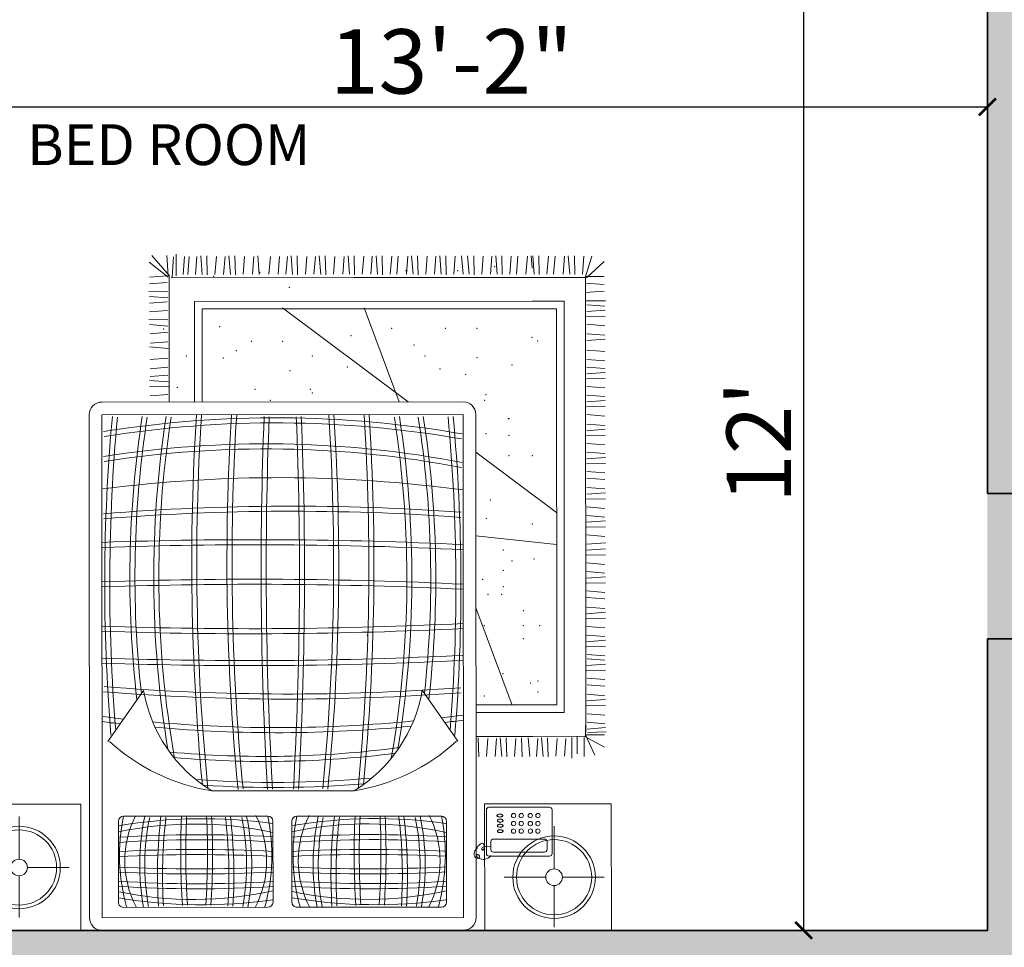
# Model space of a CAD drawing. Units: inches. Extents: x 1704 to 2334, y 1856 to 2559.
# Tile 5 of 10: x 1779 to 1925, y 2353 to 2489. Entities that reach past the tile are written whole.
import ezdxf

# ---------------------------------------------------------------- set-up
doc = ezdxf.new("R2010")
doc.units = ezdxf.units.IN
for name, color, linetype, lineweight in [('A-ANNO-DIMS', 2, 'Continuous', 18), ('A-AREA-IDEN', 7, 'Continuous', 18), ('A-WALL', 7, 'Continuous', 35), ('BEDS', 17, 'Continuous', 18)]:
    doc.layers.add(name, color=color, linetype=linetype, lineweight=lineweight)
doc.layers.add('A-WALL-PATT', color=18, linetype='Continuous', lineweight=13, true_color=0x000000)
doc.styles.get("Standard").update_dxf_attribs({"font": 'arial.ttf'})
doc.dimstyles.new('ISO-25', dxfattribs={"dimtxt": 9.5, "dimasz": 2.5, "dimexe": 1.25, "dimexo": 0.625, "dimtad": 1, "dimdec": 0, "dimlunit": 4, "dimtxsty": 'Standard', "dimblk": 'ARCHTICK', "dimcen": 2.5, "dimse1": 1, "dimse2": 1, "dimclrd": 3, "dimadec": 0, "dimazin": 0, "dimtfac": 1, "dimtdec": 0, "dimtmove": 0, "dimatfit": 3, "dimfxl": 1, "dimarcsym": 0})

# ---------------------------------------------------------------- blocks, each defined once
blk = doc.blocks.new('A$C77DF40FE')
for p, q in [((0.5, 2.6723), (0, 2.6723)), ((0, 2.6723), (0, 2.1723)), ((0.226, 2.4949), (0.226, 2.6594)), ((0.5, 2.1723), (0.5, 2.6723)), ((0.5839, 2.6714), (2.0097, 2.6714)), ((2.0936, 2.1723), (2.0936, 2.6723)), ((2.0936, 2.6723), (2.5936, 2.6723)), ((2.5936, 2.6723), (2.5936, 2.1723)), ((0.5339, 0.6344), (0.5339, 2.6214)), ((0.5839, 2.6214), (2.0097, 2.6214)), ((0.5839, 0.6344), (0.5839, 2.6214)), ((2.0097, 2.6214), (2.0097, 0.6344)), ((2.0597, 2.6214), (2.0597, 0.6344)), ((2.3379, 2.4554), (2.3379, 2.6199)), ((1.2408, 2.5803), (0.6708, 2.5803)), ((1.9255, 2.5803), (1.3555, 2.5803)), ((0.6508, 2.5603), (0.6508, 2.2403)), ((1.2608, 2.2403), (1.2608, 2.5603)), ((1.3355, 2.5603), (1.3355, 2.2403)), ((1.9455, 2.2403), (1.9455, 2.5603)), ((0.0287, 2.4621), (0.1932, 2.4621)), ((0.2588, 2.4621), (0.4233, 2.4621)), ((0.226, 2.261), (0.226, 2.4293)), ((2.3051, 2.4226), (2.1406, 2.4226)), ((2.5352, 2.4226), (2.3707, 2.4226)), ((0.4828, 2.3788, 10.4), (0.2438, 2.3788, 10.4)), ((0.4809, 2.3823), (0.4746, 2.3757)), ((0.4873, 2.387), (0.4809, 2.3823)), ((0.4937, 2.3899), (0.4873, 2.387)), ((0.5, 2.3914), (0.4937, 2.3899)), ((0.506, 2.3917), (0.5, 2.3914)), ((0.5117, 2.391), (0.506, 2.3917)), ((0.5168, 2.3897), (0.5117, 2.391)), ((0.5212, 2.3878), (0.5168, 2.3897)), ((0.5205, 2.3816), (0.5202, 2.3804)), ((0.5202, 2.3804), (0.5202, 2.379)), ((0.5202, 2.379), (0.5206, 2.3777)), ((0.521, 2.3828), (0.5205, 2.3816)), ((0.5206, 2.3777), (0.5213, 2.3764)), ((0.5219, 2.3839), (0.521, 2.3828)), ((0.5248, 2.3858), (0.5212, 2.3878)), ((0.5213, 2.3764), (0.5224, 2.3752)), ((0.523, 2.3849), (0.5219, 2.3839)), ((0.5224, 2.3752), (0.5237, 2.374)), ((0.5244, 2.3856), (0.523, 2.3849)), ((0.5237, 2.374), (0.5252, 2.3731)), ((0.5261, 2.3861), (0.5244, 2.3856)), ((0.5277, 2.3836), (0.5248, 2.3858)), ((0.5252, 2.3731), (0.5268, 2.3723)), ((0.5279, 2.3864), (0.5261, 2.3861)), ((0.5268, 2.3723), (0.5283, 2.3719)), ((0.5298, 2.3813), (0.5277, 2.3836)), ((0.5298, 2.3864), (0.5279, 2.3864)), ((0.5283, 2.3719), (0.5297, 2.3717)), ((0.5297, 2.3717), (0.531, 2.372)), ((0.5318, 2.3861), (0.5298, 2.3864)), ((0.5313, 2.3792), (0.5298, 2.3813)), ((0.531, 2.372), (0.5319, 2.3726)), ((0.5322, 2.3771), (0.5313, 2.3792)), ((0.5338, 2.3855), (0.5318, 2.3861)), ((0.5319, 2.3726), (0.5325, 2.3738)), ((0.5326, 2.3753), (0.5322, 2.3771)), ((0.5325, 2.3738), (0.5326, 2.3753)), ((0.5356, 2.3846), (0.5338, 2.3855)), ((0.5373, 2.3832), (0.5356, 2.3846)), ((0.5387, 2.3815), (0.5373, 2.3832)), ((0.5399, 2.3794), (0.5387, 2.3815)), ((0.5407, 2.377), (0.5399, 2.3794)), ((0.5412, 2.3743), (0.5407, 2.377)), ((0.5414, 2.3715), (0.5412, 2.3743)), ((0.5413, 2.3686), (0.5414, 2.3715)), ((2.3379, 2.2215), (2.3379, 2.3898)), ((0.2338, 2.3688, 10.4), (0.2338, 2.1957, 10.4)), ((0.2538, 2.353, 10.4), (0.2538, 2.3215, 10.4)), ((0.4656, 2.363, 10.4), (0.2638, 2.363, 10.4)), ((0.4756, 2.3215, 10.4), (0.4756, 2.353, 10.4)), ((0.4767, 2.3409), (0.4876, 2.34)), ((0.4876, 2.34), (0.4961, 2.3402)), ((0.4928, 2.1957, 10.4), (0.4928, 2.3688, 10.4)), ((0.4961, 2.3402), (0.5023, 2.3413)), ((0.502, 2.3463), (0.5017, 2.3431)), ((0.5017, 2.3431), (0.5018, 2.3398)), ((0.5018, 2.3398), (0.5023, 2.3365)), ((0.5026, 2.3491), (0.502, 2.3463)), ((0.5023, 2.3413), (0.5067, 2.3431)), ((0.5023, 2.3365), (0.5031, 2.3334)), ((0.5035, 2.3514), (0.5026, 2.3491)), ((0.5031, 2.3334), (0.5043, 2.3309)), ((0.5047, 2.3531), (0.5035, 2.3514)), ((0.5059, 2.3542), (0.5047, 2.3531)), ((0.5073, 2.3548), (0.5059, 2.3542)), ((0.5067, 2.3431), (0.5095, 2.3452)), ((0.5086, 2.3549), (0.5073, 2.3548)), ((0.5097, 2.3544), (0.5086, 2.3549)), ((0.5095, 2.3452), (0.511, 2.3475)), ((0.5107, 2.3534), (0.5097, 2.3544)), ((0.5113, 2.3518), (0.5107, 2.3534)), ((0.511, 2.3475), (0.5115, 2.3498)), ((0.5115, 2.3498), (0.5113, 2.3518)), ((0.5163, 2.3304), (0.5193, 2.3325)), ((0.5193, 2.3325), (0.5222, 2.3349)), ((0.5222, 2.3349), (0.5249, 2.3374)), ((0.5249, 2.3374), (0.5271, 2.3398)), ((0.5271, 2.3398), (0.5288, 2.3419)), ((0.5288, 2.3419), (0.5299, 2.3436)), ((0.5299, 2.3436), (0.5305, 2.3449)), ((0.53, 2.3482), (0.5302, 2.3488)), ((0.5301, 2.3477), (0.53, 2.3482)), ((0.5303, 2.3472), (0.5301, 2.3477)), ((0.5302, 2.3488), (0.5308, 2.3495)), ((0.5306, 2.3466), (0.5303, 2.3472)), ((0.5305, 2.3449), (0.5307, 2.3459)), ((0.5307, 2.3459), (0.5306, 2.3466)), ((0.5308, 2.3495), (0.5317, 2.3504)), ((0.5317, 2.3504), (0.5329, 2.3515)), ((0.5329, 2.3515), (0.5342, 2.3528)), ((0.5342, 2.3528), (0.5356, 2.3543)), ((0.5356, 2.3543), (0.537, 2.3561)), ((0.537, 2.3561), (0.5383, 2.3581)), ((0.5383, 2.3581), (0.5394, 2.3604)), ((0.5394, 2.3604), (0.5403, 2.3629)), ((0.5403, 2.3629), (0.5409, 2.3657)), ((0.5409, 2.3657), (0.5413, 2.3686)), ((0.2638, 2.3115, 10.4), (0.4656, 2.3115, 10.4)), ((0.5043, 2.3309), (0.506, 2.329)), ((0.506, 2.329), (0.5081, 2.328)), ((0.5081, 2.328), (0.5106, 2.328)), ((0.5106, 2.328), (0.5134, 2.3288)), ((0.5134, 2.3288), (0.5163, 2.3304)), ((0.6708, 2.2203), (1.2408, 2.2203)), ((1.3555, 2.2203), (1.9255, 2.2203)), ((0.2438, 2.1857, 10.4), (0.4828, 2.1857, 10.4)), ((0, 2.1723), (0.5, 2.1723)), ((2.5936, 2.1723), (2.0936, 2.1723)), ((1.5773, 2.1205), (1.0147, 2.1205)), ((0.1072, 1.986), (0.1072, 1.911)), ((0.1554, 1.9914), (0.1554, 1.911)), ((0.1792, 1.9138), (0.1849, 1.9847)), ((0.2134, 1.9138), (0.219, 1.9847)), ((0.251, 1.9118), (0.2494, 1.9865)), ((0.2748, 1.9118), (0.2691, 1.9849)), ((0.2899, 1.9138), (0.2956, 1.9847)), ((0.3277, 1.9118), (0.3219, 1.9849)), ((0.3539, 1.9118), (0.3522, 1.9865)), ((0.3766, 1.9138), (0.3822, 1.9847)), ((0.4142, 1.9118), (0.4126, 1.9865)), ((0.438, 1.9118), (0.4323, 1.9849)), ((0.4531, 1.9138), (0.4588, 1.9847)), ((0.4873, 1.9138), (0.493, 1.9847)), ((0.5249, 1.9118), (0.5233, 1.9865)), ((0.1072, 1.9057), (0.0269, 1.9485)), ((0.0644, 1.9807), (0.1019, 1.9003)), ((0.134, 1.9753), (0.134, 1.9057)), ((0.3112, 1.9057), (0.1019, 1.9057)), ((0.1019, 1.9057), (0.1019, 1.8628)), ((0.5301, 1.9057), (0.3112, 1.9057)), ((0.6051, 1.925), (0.7457, 1.7234)), ((1.9869, 1.925), (1.8463, 1.7234)), ((0.0195, 1.8887), (0.0942, 1.8903)), ((0.0227, 1.8712), (0.0957, 1.8769)), ((0.1019, 1.9003), (0.0269, 1.9003)), ((0.1002, 1.8885), (0.1002, 0.0935)), ((0.0247, 1.8561), (0.0955, 1.8504)), ((0.0247, 1.8219), (0.0955, 1.8163)), ((0.3112, 1.8116), (0.1852, 1.8116)), ((0.1852, 1.8116), (0.1852, 0.187)), ((0.5339, 1.8116), (0.3112, 1.8116)), ((0.0227, 1.7843), (0.0974, 1.786)), ((0.0227, 1.7605), (0.0957, 1.7662)), ((0.3112, 1.7816), (0.2152, 1.7816)), ((0.2152, 1.7816), (0.2152, 0.217)), ((0.5339, 1.7816), (0.3112, 1.7816)), ((0.3909, 1.7821), (0.5339, 1.398)), ((0.0247, 1.7454), (0.0955, 1.7397)), ((0.0247, 1.708), (0.0955, 1.7023)), ((0.0247, 1.6819), (0.0955, 1.6762)), ((0.0227, 1.6443), (0.0974, 1.6459)), ((0.0227, 1.6205), (0.0957, 1.6262)), ((0.0247, 1.6054), (0.0955, 1.5997)), ((0.0247, 1.5881), (0.0955, 1.5824)), ((0.0227, 1.5505), (0.0974, 1.5521)), ((0.0227, 1.5266), (0.0957, 1.5324)), ((0.0247, 1.5116), (0.0955, 1.5059)), ((0.0247, 1.4774), (0.0955, 1.4717)), ((0.0227, 1.4397), (0.0974, 1.4414)), ((0.0227, 1.4159), (0.0957, 1.4217)), ((0.0247, 1.4008), (0.0955, 1.3952)), ((0.0247, 1.3634), (0.0955, 1.3577)), ((0.0247, 1.3374), (0.0955, 1.3317)), ((0.0227, 1.2997), (0.0974, 1.3014)), ((0.0227, 1.2759), (0.0957, 1.2816)), ((0.0247, 1.2608), (0.0955, 1.2551)), ((0.0247, 1.2266), (0.0955, 1.221)), ((0.0227, 1.189), (0.0974, 1.1906)), ((0.0227, 1.1652), (0.0957, 1.1709)), ((0.0227, 1.1414), (0.0957, 1.1471)), ((0.5339, 1.1132), (0.2152, 1.1479)), ((0.0247, 1.1163), (0.0955, 1.1106)), ((0.0227, 1.0786), (0.0974, 1.0803)), ((0.0227, 1.0548), (0.0957, 1.0606)), ((0.0247, 1.0397), (0.0955, 1.0341)), ((0.5339, 0.7837), (0.2152, 1.0221)), ((0.0247, 1.0055), (0.0955, 0.9999)), ((0.0227, 0.9679), (0.0974, 0.9696)), ((0.0227, 0.9441), (0.0957, 0.9498)), ((0.0247, 0.929), (0.0955, 0.9233)), ((0.0247, 0.8916), (0.0955, 0.8859)), ((0.0247, 0.8655), (0.0955, 0.8599)), ((0.0227, 0.8279), (0.0974, 0.8295)), ((0.0227, 0.8041), (0.0957, 0.8098)), ((0.0247, 0.789), (0.0955, 0.7833)), ((0.0247, 0.7548), (0.0955, 0.7491)), ((0.0227, 0.7172), (0.0974, 0.7188)), ((0.0227, 0.6933), (0.0957, 0.6991)), ((0.0247, 0.6783), (0.0955, 0.6726)), ((0.0247, 0.6408), (0.0955, 0.6352)), ((2.0097, 0.6344), (0.5839, 0.6344)), ((0.0227, 0.6032), (0.0974, 0.6048)), ((0.0227, 0.5794), (0.0957, 0.5851)), ((2.0097, 0.5844), (0.5839, 0.5844)), ((1.2963, 0.2134), (0.8003, 0.5844)), ((0.8369, 0.5844), (0.975, 0.2134)), ((1.6139, 0.217), (1.6139, 0.5844)), ((1.6439, 0.187), (1.6439, 0.5844)), ((1.7439, 0.087), (1.7439, 0.5844)), ((0.0247, 0.5643), (0.0955, 0.5586)), ((1.8197, 0.5605), (1.7489, 0.5548)), ((0.0247, 0.5301), (0.0955, 0.5244)), ((1.8218, 0.5229), (1.7471, 0.5245)), ((0.0227, 0.4925), (0.0974, 0.4941)), ((0.0227, 0.4687), (0.0957, 0.4744)), ((1.8218, 0.499), (1.7487, 0.5048)), ((1.8197, 0.4839), (1.7489, 0.4783)), ((0.0247, 0.4536), (0.0955, 0.4479)), ((1.8197, 0.453), (1.7489, 0.4474)), ((0.0247, 0.4227), (0.0955, 0.417)), ((1.8197, 0.4168), (1.7489, 0.4111)), ((0.0247, 0.3864), (0.0955, 0.3807)), ((1.8218, 0.3671), (1.7487, 0.3728)), ((1.8197, 0.352), (1.7489, 0.3463)), ((0.0227, 0.3367), (0.0957, 0.3424)), ((0.0247, 0.3216), (0.0955, 0.3159)), ((1.8197, 0.3146), (1.7489, 0.3089)), ((0.0247, 0.2842), (0.0955, 0.2785)), ((1.7492, 0.2844), (1.8223, 0.2787)), ((0.0227, 0.2465), (0.0974, 0.2482)), ((1.7492, 0.2606), (1.824, 0.2589)), ((0.0227, 0.2227), (0.0957, 0.2285)), ((0.0247, 0.2076), (0.0955, 0.202)), ((0.2152, 0.217), (0.3112, 0.217)), ((0.3112, 0.217), (1.6139, 0.217)), ((1.7513, 0.223), (1.8221, 0.2286)), ((1.7513, 0.1888), (1.8221, 0.1944)), ((0.1019, 0.1857), (0.0216, 0.1857)), ((0.1852, 0.187), (0.3112, 0.187)), ((0.3112, 0.187), (1.6439, 0.187)), ((1.7492, 0.1737), (1.8223, 0.1679)), ((0.1019, 0.1535), (0.0269, 0.1482)), ((0.1019, 0.116), (0.0269, 0.1214)), ((1.7492, 0.1499), (1.824, 0.1482)), ((1.7513, 0.1122), (1.8221, 0.1179)), ((0.0965, 0.0946), (0.0269, 0.0303)), ((0.1019, 0.0892), (0.0269, 0.0892)), ((0.1019, 0.0946), (0.0751, 0.0089)), ((0.1002, 0.0935), (0.3112, 0.0935)), ((0.107, 0.0096), (0.1126, 0.0804)), ((0.1446, 0.0075), (0.1429, 0.0823)), ((0.1684, 0.0075), (0.1627, 0.0806)), ((0.1835, 0.0096), (0.1892, 0.0804)), ((0.2209, 0.0096), (0.2266, 0.0804)), ((0.247, 0.0096), (0.2527, 0.0804)), ((0.2846, 0.0075), (0.283, 0.0823)), ((0.3084, 0.0075), (0.3027, 0.0806)), ((0.3112, 0.0935), (1.0155, 0.0935)), ((0.3301, 0.0096), (0.3358, 0.0804)), ((0.3676, 0.0096), (0.3732, 0.0804)), ((0.3936, 0.0096), (0.3993, 0.0804)), ((0.4313, 0.0075), (0.4296, 0.0823)), ((0.4551, 0.0075), (0.4493, 0.0806)), ((0.4702, 0.0096), (0.4758, 0.0804)), ((0.5043, 0.0096), (0.51, 0.0804)), ((0.542, 0.0075), (0.5403, 0.0823)), ((0.5658, 0.0075), (0.56, 0.0806)), ((0.5896, 0.0075), (0.5838, 0.0806)), ((0.6147, 0.0096), (0.6204, 0.0804)), ((0.6523, 0.0075), (0.6507, 0.0823)), ((0.6762, 0.0075), (0.6704, 0.0806)), ((0.6912, 0.0096), (0.6969, 0.0804)), ((0.7254, 0.0096), (0.7311, 0.0804)), ((0.7631, 0.0075), (0.7614, 0.0823)), ((0.7869, 0.0075), (0.7811, 0.0806)), ((0.802, 0.0096), (0.8076, 0.0804)), ((0.8394, 0.0096), (0.8451, 0.0804)), ((0.8654, 0.0096), (0.8711, 0.0804)), ((0.9031, 0.0075), (0.9014, 0.0823)), ((0.9269, 0.0075), (0.9212, 0.0806)), ((0.942, 0.0096), (0.9477, 0.0804)), ((0.9762, 0.0096), (0.9818, 0.0804)), ((1.0138, 0.0075), (1.0122, 0.0823)), ((1.0155, 0.0935), (1.7355, 0.0935)), ((1.0376, 0.0075), (1.0319, 0.0806)), ((1.0527, 0.0096), (1.0584, 0.0804)), ((1.0901, 0.0096), (1.0958, 0.0804)), ((1.1278, 0.0075), (1.1261, 0.0823)), ((1.1516, 0.0075), (1.1459, 0.0806)), ((1.1667, 0.0096), (1.1724, 0.0804)), ((1.2009, 0.0096), (1.2065, 0.0804)), ((1.2385, 0.0075), (1.2368, 0.0823)), ((1.2623, 0.0075), (1.2566, 0.0806)), ((1.2774, 0.0096), (1.2831, 0.0804)), ((1.3083, 0.0096), (1.314, 0.0804)), ((1.3446, 0.0096), (1.3503, 0.0804)), ((1.3943, 0.0075), (1.3885, 0.0806)), ((1.4094, 0.0096), (1.415, 0.0804)), ((1.4468, 0.0096), (1.4525, 0.0804)), ((1.4844, 0.0075), (1.4828, 0.0823)), ((1.5083, 0.0075), (1.5025, 0.0806)), ((1.5233, 0.0096), (1.529, 0.0804)), ((1.5575, 0.0096), (1.5632, 0.0804)), ((1.5951, 0.0075), (1.5935, 0.0823)), ((1.619, 0.0075), (1.6132, 0.0806)), ((1.6341, 0.0096), (1.6397, 0.0804)), ((1.665, 0.0096), (1.6706, 0.0804)), ((1.6831, 0.0096), (1.6888, 0.0804)), ((1.7162, 0.0857), (1.7162, 0)), ((1.7323, 0.0911), (1.7269, 0.0107)), ((1.743, 0.0857), (1.8126, 0.0054)), ((1.7483, 0.0911), (1.8233, 0.0322)), ((1.7483, 0.0857), (1.7537, 0.0054)), ((1.7513, 0.0858), (1.8221, 0.0915)), ((0.3151, 0.0075), (0.3112, 0.0565))]:
    blk.add_line(p, q)
for centre, radius in [((0.226, 2.4621), 0.1629), ((0.226, 2.4621), 0.1484), ((2.3379, 2.4226), 0.1629), ((2.3379, 2.4226), 0.1484), ((0.226, 2.4621), 0.0328), ((2.3379, 2.4226), 0.0328), ((0.2896, 2.2801, 10.4), 0.00858), ((0.2896, 2.25, 10.4), 0.00858), ((0.3196, 2.2801, 10.4), 0.00858), ((0.3196, 2.25, 10.4), 0.00858), ((0.3554, 2.2801, 10.4), 0.00858), ((0.3554, 2.25, 10.4), 0.00858), ((0.3855, 2.2801, 10.4), 0.00858), ((0.3855, 2.25, 10.4), 0.00858), ((0.2896, 2.2186, 10.4), 0.00858), ((0.3196, 2.2186, 10.4), 0.00858), ((0.3554, 2.2186, 10.4), 0.00858), ((0.3855, 2.2186, 10.4), 0.00858)]:
    blk.add_circle(centre, radius)
for centre, radius, start, end in [((0.5839, 2.6214), 0.05, 90, 180), ((2.0097, 2.6214), 0.05, 0, 90), ((0.6708, 2.5603), 0.02, 90, 180), ((0.9287, 0.5819), 1.9884, 80.4201, 97.9672), ((1.4247, 2.3742), 0.7696, 164.6112, 191.5679), ((1.0701, 2.3966), 0.3942, 152.5365, 206.92), ((1.6628, 2.4129), 0.928, 169.6087, 191.899), ((1.6628, 2.4129), 0.908, 169.6087, 191.899), ((2.7571, 2.4533), 1.9523, 176.3947, 186.8195), ((2.7571, 2.4533), 1.9323, 176.3947, 186.8195), ((3.9259, 2.3685), 3.0367, 176.1432, 182.775), ((3.9259, 2.3685), 3.0167, 176.1432, 182.775), ((-2.0216, 2.3685), 3.0167, 357.225, 3.8568), ((-2.0216, 2.3685), 3.0367, 357.225, 3.8568), ((-0.8455, 2.4533), 1.9323, 353.1805, 3.6053), ((-0.8455, 2.4533), 1.9523, 353.1805, 3.6053), ((0.2489, 2.4129), 0.908, 348.101, 10.3913), ((0.2489, 2.4129), 0.928, 348.101, 10.3913), ((0.8416, 2.3966), 0.3942, 333.08, 27.4635), ((0.4869, 2.3742), 0.7696, 348.4321, 15.3888), ((1.2408, 2.5603), 0.02, 0, 90), ((1.3555, 2.5603), 0.02, 90, 180), ((1.6135, 0.5819), 1.9884, 80.4201, 97.9672), ((2.1094, 2.3742), 0.7696, 164.6112, 191.5679), ((1.7548, 2.3966), 0.3942, 152.5365, 206.92), ((2.3475, 2.4129), 0.928, 169.6087, 191.899), ((2.3475, 2.4129), 0.908, 169.6087, 191.899), ((3.4419, 2.4533), 1.9523, 176.3947, 186.8195), ((3.4419, 2.4533), 1.9323, 176.3947, 186.8195), ((4.6106, 2.3685), 3.0367, 176.1432, 182.775), ((4.6106, 2.3685), 3.0167, 176.1432, 182.775), ((-1.3369, 2.3685), 3.0167, 357.225, 3.8568), ((-1.3369, 2.3685), 3.0367, 357.225, 3.8568), ((-0.1608, 2.4533), 1.9323, 353.1805, 3.6053), ((-0.1608, 2.4533), 1.9523, 353.1805, 3.6053), ((0.9336, 2.4129), 0.908, 348.101, 10.3913), ((0.9336, 2.4129), 0.928, 348.101, 10.3913), ((1.5263, 2.3966), 0.3942, 333.08, 27.4635), ((1.1716, 2.3742), 0.7696, 348.4321, 15.3888), ((1.9255, 2.5603), 0.02, 0, 90), ((0.9635, 1.1066), 1.4427, 78.1527, 102.4906), ((1.6482, 1.1066), 1.4427, 78.1527, 102.4906), ((0.9445, -2.3575), 4.8647, 86.2671, 93.4563), ((1.6292, -2.3575), 4.8647, 86.2671, 93.4563), ((0.9561, -3.928), 6.3765, 87.24779, 92.75221), ((0.9445, -2.3575), 4.8447, 86.2671, 93.4563), ((1.6408, -3.928), 6.3765, 87.24779, 92.75221), ((1.6292, -2.3575), 4.8447, 86.2671, 93.4563), ((0.9561, -3.928), 6.3565, 87.24779, 92.75221), ((1.6408, -3.928), 6.3565, 87.24779, 92.75221), ((0.2438, 2.3688, 10.4), 0.01, 90, 180), ((0.4828, 2.3688, 10.4), 0.01, 0, 90), ((0.9561, 8.7285), 6.3565, 267.24779, 272.75221), ((1.6408, 8.7285), 6.3565, 267.24779, 272.75221), ((0.2638, 2.353, 10.4), 0.01, 90, 180), ((0.4656, 2.353, 10.4), 0.01, 0, 90), ((0.9561, 8.7285), 6.3765, 267.24779, 272.75221), ((1.6408, 8.7285), 6.3765, 267.24779, 272.75221), ((0.2638, 2.3215, 10.4), 0.01, 180, 270), ((0.4656, 2.3215, 10.4), 0.01, 270, 0), ((0.9445, 7.158), 4.8647, 266.5437, 273.7329), ((0.9445, 7.158), 4.8447, 266.5437, 273.7329), ((1.6292, 7.158), 4.8647, 266.5437, 273.7329), ((1.6292, 7.158), 4.8447, 266.5437, 273.7329), ((0.43, 2.2801, 10.4), 0.00304, 140.3607, 180), ((0.43, 2.2801, 10.4), 0.00304, 180, 219.6393), ((0.43, 2.2586, 10.4), 0.00304, 140.3607, 180), ((0.43, 2.2586, 10.4), 0.00304, 180, 219.6393), ((0.434, 2.2768, 10.4), 0.00822, 116.5651, 140.3607), ((0.434, 2.2834, 10.4), 0.00822, 219.6393, 243.4349), ((0.434, 2.2553, 10.4), 0.00822, 116.5651, 140.3607), ((0.434, 2.2619, 10.4), 0.00822, 219.6393, 243.4349), ((0.4367, 2.2714, 10.4), 0.0142, 101.7009, 116.5651), ((0.4367, 2.2887, 10.4), 0.0142, 243.4349, 258.2991), ((0.4367, 2.25, 10.4), 0.0142, 101.7009, 116.5651), ((0.4367, 2.2673, 10.4), 0.0142, 243.4349, 258.2991), ((0.4384, 2.263, 10.4), 0.0228, 90, 101.7009), ((0.4384, 2.2972, 10.4), 0.0228, 258.2991, 270), ((0.4384, 2.2415, 10.4), 0.0228, 90, 101.7009), ((0.4384, 2.263, 10.4), 0.0228, 78.2991, 90), ((0.4384, 2.2972, 10.4), 0.0228, 270, 281.7009), ((0.4384, 2.2415, 10.4), 0.0228, 78.2991, 90), ((0.4402, 2.2714, 10.4), 0.0142, 63.4349, 78.2991), ((0.4402, 2.2887, 10.4), 0.0142, 281.7009, 296.5651), ((0.4402, 2.25, 10.4), 0.0142, 63.4349, 78.2991), ((0.4402, 2.2673, 10.4), 0.0142, 281.7009, 296.5651), ((0.4428, 2.2768, 10.4), 0.00822, 39.6393, 63.4349), ((0.4428, 2.2834, 10.4), 0.00822, 296.5651, 320.3607), ((0.4428, 2.2553, 10.4), 0.00822, 39.6393, 63.4349), ((0.4428, 2.2619, 10.4), 0.00822, 296.5651, 320.3607), ((0.4468, 2.2801, 10.4), 0.00304, 0, 39.6393), ((0.4468, 2.2801, 10.4), 0.00304, 320.3607, 0), ((0.4468, 2.2586, 10.4), 0.00304, 0, 39.6393), ((0.4468, 2.2586, 10.4), 0.00304, 320.3607, 0), ((0.9635, 3.6939), 1.4427, 257.5094, 281.8473), ((0.9287, 4.2186), 1.9884, 262.0328, 279.5799), ((1.6482, 3.6939), 1.4427, 257.5094, 281.8473), ((1.6135, 4.2186), 1.9884, 262.0328, 279.5799), ((0.43, 2.2386, 10.4), 0.00304, 140.3607, 180), ((0.43, 2.2386, 10.4), 0.00304, 180, 219.6393), ((0.434, 2.2353, 10.4), 0.00822, 116.5651, 140.3607), ((0.434, 2.2419, 10.4), 0.00822, 219.6393, 243.4349), ((0.4314, 2.2186, 10.4), 0.00304, 140.3607, 180), ((0.4314, 2.2186, 10.4), 0.00304, 180, 219.6393), ((0.4354, 2.2153, 10.4), 0.00822, 116.5651, 140.3607), ((0.4354, 2.2219, 10.4), 0.00822, 219.6393, 243.4349), ((0.4367, 2.23, 10.4), 0.0142, 101.7009, 116.5651), ((0.4367, 2.2472, 10.4), 0.0142, 243.4349, 258.2991), ((0.4381, 2.2099, 10.4), 0.0142, 101.7009, 116.5651), ((0.4384, 2.2757, 10.4), 0.0228, 258.2991, 270), ((0.4384, 2.2215, 10.4), 0.0228, 90, 101.7009), ((0.4384, 2.2557, 10.4), 0.0228, 258.2991, 270), ((0.4398, 2.2015, 10.4), 0.0228, 90, 101.7009), ((0.4384, 2.2757, 10.4), 0.0228, 270, 281.7009), ((0.4384, 2.2215, 10.4), 0.0228, 78.2991, 90), ((0.4384, 2.2557, 10.4), 0.0228, 270, 281.7009), ((0.4398, 2.2015, 10.4), 0.0228, 78.2991, 90), ((0.4402, 2.23, 10.4), 0.0142, 63.4349, 78.2991), ((0.4402, 2.2472, 10.4), 0.0142, 281.7009, 296.5651), ((0.4416, 2.2099, 10.4), 0.0142, 63.4349, 78.2991), ((0.4428, 2.2353, 10.4), 0.00822, 39.6393, 63.4349), ((0.4428, 2.2419, 10.4), 0.00822, 296.5651, 320.3607), ((0.4443, 2.2153, 10.4), 0.00822, 39.6393, 63.4349), ((0.4443, 2.2219, 10.4), 0.00822, 296.5651, 320.3607), ((0.4468, 2.2386, 10.4), 0.00304, 0, 39.6393), ((0.4468, 2.2386, 10.4), 0.00304, 320.3607, 0), ((0.4483, 2.2186, 10.4), 0.00304, 0, 39.6393), ((0.4483, 2.2186, 10.4), 0.00304, 320.3607, 0), ((0.6708, 2.2403), 0.02, 180, 270), ((1.2408, 2.2403), 0.02, 270, 0), ((1.3555, 2.2403), 0.02, 180, 270), ((1.9255, 2.2403), 0.02, 270, 0), ((0.2438, 2.1957, 10.4), 0.01, 180, 270), ((0.4381, 2.2272, 10.4), 0.0142, 243.4349, 258.2991), ((0.4398, 2.2357, 10.4), 0.0228, 258.2991, 270), ((0.4398, 2.2357, 10.4), 0.0228, 270, 281.7009), ((0.4416, 2.2272, 10.4), 0.0142, 281.7009, 296.5651), ((0.4828, 2.1957, 10.4), 0.01, 270, 0), ((1.1396, 1.3485), 0.782, 99.1908, 132.5116), ((1.3217, 1.6229), 0.5847, 121.6676, 170.1065), ((10.1174, 1.2237), 9.161, 174.43278, 183.67204), ((1.3248, -2.1722), 4.2793, 86.1532, 94.7091), ((10.2564, 1.2237), 9.181, 174.43278, 183.67204), ((10.2564, 1.2237), 9.161, 174.43278, 183.67204), ((16.3019, 1.253), 15.0916, 176.72768, 182.32074), ((16.3019, 1.253), 15.0716, 176.72768, 182.32074), ((-13.7099, 1.253), 15.0716, 357.67926, 3.27232), ((-13.7099, 1.253), 15.0916, 357.67926, 3.27232), ((-7.6644, 1.2237), 9.161, 356.32796, 5.56722), ((-7.6644, 1.2237), 9.181, 356.32796, 5.56722), ((1.2703, 1.6229), 0.5847, 9.8935, 58.3324), ((1.4523, 1.3485), 0.782, 47.4884, 80.8092), ((-7.5254, 1.2237), 9.161, 356.32796, 5.55658), ((10.1174, 1.2237), 9.181, 174.54912, 183.67204), ((1.3248, -2.1722), 4.2593, 85.7473, 95.1159), ((-7.5254, 1.2237), 9.181, 356.32796, 5.45088), ((4.947, 1.2796), 4.1406, 170.0939, 188.8179), ((1.3657, -2.1044), 4.0888, 84.7053, 97.4283), ((1.3657, -2.1044), 4.1088, 84.9619, 97.1707), ((-2.355, 1.2796), 4.1406, 351.1821, 9.9061), ((4.947, 1.2796), 4.1606, 170.6272, 188.8179), ((-2.355, 1.2796), 4.1606, 351.1821, 9.3728), ((7.8077, 1.3061), 7.2149, 175.27403, 185.28261), ((7.8077, 1.3061), 7.1949, 175.41729, 185.28261), ((1.3142, -3.5764), 5.4471, 84.7792, 95.6214), ((1.3142, -3.5764), 5.4671, 84.8953, 95.5052), ((-5.2157, 1.3061), 7.1949, 354.71739, 4.58271), ((-5.2157, 1.3061), 7.2149, 354.71739, 4.72597), ((1.3142, -3.5764), 5.4671, 96.9078, 97.6924), ((1.3142, -3.5764), 5.4471, 96.796, 97.6924), ((1.3142, -3.5764), 5.4471, 82.7025, 83.5609), ((1.3142, -3.5764), 5.4671, 82.7025, 83.4474), ((1.2659, -7.4764), 9.2344, 85.41732, 94.18368), ((4.8527, 1.2796), 4.1606, 173.3677, 188.8179), ((-2.2608, 1.2796), 4.1606, 351.1821, 6.6323), ((1.2659, -7.4764), 9.2144, 85.41732, 94.18368), ((4.8527, 1.2796), 4.1406, 173.6812, 188.8179), ((-2.2608, 1.2796), 4.1406, 351.1821, 6.3188), ((1.4138, -15.5462), 17.172, 88.01473, 92.775), ((1.4138, -15.5462), 17.152, 88.01473, 92.775), ((1.4138, -15.6721), 17.172, 88.01473, 92.775), ((1.4138, -15.6721), 17.152, 88.01473, 92.775), ((1.4138, 18.4566), 17.152, 267.225, 271.98527), ((1.4138, 18.4566), 17.172, 267.225, 271.98527), ((1.4138, 18.3004), 17.152, 267.225, 271.98527), ((1.4138, 18.3004), 17.172, 267.225, 271.98527), ((1.2659, 10.2305), 9.2344, 265.81632, 274.58268), ((1.2659, 10.2305), 9.2144, 265.81632, 274.58268), ((1.3142, 6.3306), 5.4471, 262.3076, 277.2975), ((1.3657, 4.8586), 4.1088, 259.0794, 278.9327), ((1.3657, 4.8586), 4.0888, 259.0794, 278.9327), ((1.3248, 4.9264), 4.2793, 260.0761, 279.1287), ((1.3248, 4.9264), 4.2593, 260.0761, 279.1287), ((0.5839, 0.6344), 0.05, 180, 270), ((2.0097, 0.6344), 0.05, 270, 0)]:
    blk.add_arc(centre, radius, start, end)
for p in [(0.2895, 1.7311), (0.5004, 1.7457), (0.2895, 1.6873), (0.3179, 1.6946), (0.4274, 1.6581), (0.3471, 1.5195), (0.9622, 1.5058), (0.2822, 1.4684), (0.3471, 1.4684), (0.5004, 1.4684), (0.3471, 1.41), (0.4326, 1.3443), (0.4858, 1.3444), (0.4253, 1.3151), (0.5077, 1.286), (0.4253, 1.2495), (0.3041, 1.2057), (0.3909, 1.213), (0.4253, 1.1692), (0.3106, 1.0671), (0.4931, 1.0452), (0.4765, 0.9722), (0.3114, 0.7971), (0.4034, 0.7971), (0.4034, 0.7169), (0.4931, 0.7096), (0.4034, 0.6512), (0.4055, 0.6512), (0.4931, 0.5564), (0.4984, 0.5782), (1.1794, 0.5491), (1.3453, 0.5782), (1.1867, 0.5345), (1.4058, 0.5345), (1.7124, 0.5272), (0.5734, 0.4761), (0.3909, 0.4396), (0.6757, 0.4542), (1.0407, 0.4469), (1.2671, 0.4615), (0.5296, 0.4104), (0.7341, 0.4032), (1.1794, 0.4032), (1.5299, 0.4104), (1.6759, 0.4032), (0.7779, 0.3594), (1.4788, 0.3813), (0.2895, 0.3448), (0.3114, 0.3302), (1.0261, 0.3229), (1.2963, 0.3448), (1.4204, 0.3448), (0.5296, 0.2937), (0.6538, 0.2937), (0.8655, 0.2937), (1.5445, 0.2864), (1.7652, 0.2958), (1.2693, 0.1315), (1.5686, 0.0878), (0.4588, 0.0513), (0.6049, 0.0659), (0.8093, 0.0659), (1.3861, 0.0732)]:
    blk.add_point(p)
blk = doc.blocks.new('_ArchTick')
at = {"color": 0, "linetype": 'ByBlock', "const_width": 0.15}
blk.add_lwpolyline([(-0.5, -0.5), (0.5, 0.5)], dxfattribs=at)
blk = doc.blocks.new('*D11')
at = {"layer": 'A-ANNO-DIMS', "color": 0, "lineweight": -2, "transparency": 16777216}
blk.add_line((1894.94, 2355.04), (1894.94, 2499.04), dxfattribs=at)
at = {"layer": 'Defpoints', "color": 0, "transparency": 16777216}
for p in [(1894.94, 2499.04), (1905.46, 2499.04), (1905.46, 2355.04)]:
    blk.add_point(p, dxfattribs=at)
at = {"layer": 'A-ANNO-DIMS', "color": 0, "lineweight": -2, "transparency": 16777216, "xscale": 2.5, "yscale": 2.5, "zscale": 2.5}
for p, rotation in [((1894.94, 2499.04), 90), ((1894.94, 2355.04), 270)]:
    blk.add_blockref('_ArchTick', p, dxfattribs=dict(at, rotation=rotation))
at = {"layer": 'A-ANNO-DIMS', "color": 0, "transparency": 16777216, "insert": (1889.55, 2427.04), "char_height": 9.5, "attachment_point": 5, "rotation": 90}
blk.add_mtext("12'", dxfattribs=at)
blk = doc.blocks.new('*D12')
at = {"layer": 'A-ANNO-DIMS', "color": 0, "lineweight": -2, "transparency": 16777216}
blk.add_line((1764.01, 2476.46), (1922.01, 2476.46), dxfattribs=at)
at = {"layer": 'Defpoints', "color": 0, "transparency": 16777216}
for p in [(1922.01, 2476.46), (1764.01, 2468.82), (1922.01, 2468.82)]:
    blk.add_point(p, dxfattribs=at)
at = {"layer": 'A-ANNO-DIMS', "color": 0, "lineweight": -2, "transparency": 16777216, "xscale": 2.5, "yscale": 2.5, "zscale": 2.5, "rotation": 180}
blk.add_blockref('_ArchTick', (1764.01, 2476.46), dxfattribs=at)
at = {"layer": 'A-ANNO-DIMS', "color": 0, "lineweight": -2, "transparency": 16777216, "xscale": 2.5, "yscale": 2.5, "zscale": 2.5}
blk.add_blockref('_ArchTick', (1922.01, 2476.46), dxfattribs=at)
at = {"layer": 'A-ANNO-DIMS', "color": 0, "transparency": 16777216, "insert": (1843.01, 2481.94), "char_height": 9.5, "attachment_point": 5}
blk.add_mtext('13\'-2"', dxfattribs=at)
blk = doc.blocks.new('*D43')
at = {"layer": 'A-ANNO-DIMS', "color": 3, "lineweight": -2, "transparency": 16777216}
blk.add_line((1764.01, 2539.39), (1796.13, 2539.39), dxfattribs=at)
at = {"layer": 'Defpoints', "color": 0, "transparency": 16777216}
for p in [(1796.13, 2539.39), (1764.01, 2148.04), (1796.13, 2148.04)]:
    blk.add_point(p, dxfattribs=at)
at = {"layer": 'A-ANNO-DIMS', "color": 3, "lineweight": -2, "transparency": 16777216, "xscale": 2.5, "yscale": 2.5, "zscale": 2.5, "rotation": 180}
blk.add_blockref('_ArchTick', (1764.01, 2539.39), dxfattribs=at)
at = {"layer": 'A-ANNO-DIMS', "color": 3, "lineweight": -2, "transparency": 16777216, "xscale": 2.5, "yscale": 2.5, "zscale": 2.5}
blk.add_blockref('_ArchTick', (1796.13, 2539.39), dxfattribs=at)
at = {"layer": 'A-ANNO-DIMS', "color": 0, "transparency": 16777216, "insert": (1780.07, 2544.86), "char_height": 9.5, "attachment_point": 5}
blk.add_mtext('2\'-8"', dxfattribs=at)
blk = doc.blocks.new('*D48')
at = {"layer": 'A-ANNO-DIMS', "color": 3, "lineweight": -2, "transparency": 16777216}
for p, q in [((1764.01, 2539.39), (1799.73, 2539.39)), ((1799.73, 2539.39), (1858.41, 2539.39))]:
    blk.add_line(p, q, dxfattribs=at)
at = {"layer": 'Defpoints', "color": 0, "transparency": 16777216}
for p in [(1799.73, 2539.39), (1764.01, 2200.93), (1799.73, 2200.93)]:
    blk.add_point(p, dxfattribs=at)
at = {"layer": 'A-ANNO-DIMS', "color": 3, "lineweight": -2, "transparency": 16777216, "xscale": 2.5, "yscale": 2.5, "zscale": 2.5, "rotation": 180}
blk.add_blockref('_ArchTick', (1764.01, 2539.39), dxfattribs=at)
at = {"layer": 'A-ANNO-DIMS', "color": 3, "lineweight": -2, "transparency": 16777216, "xscale": 2.5, "yscale": 2.5, "zscale": 2.5}
blk.add_blockref('_ArchTick', (1799.73, 2539.39), dxfattribs=at)
at = {"layer": 'A-ANNO-DIMS', "color": 0, "transparency": 16777216, "insert": (1830.32, 2544.93), "char_height": 9.5, "attachment_point": 5}
blk.add_mtext('2\'-11 1/2"', dxfattribs=at)
blk = doc.blocks.new('*D53')
at = {"layer": 'A-ANNO-DIMS', "color": 3, "lineweight": -2, "transparency": 16777216}
for p, q in [((1764.01, 1864.5), (1798.75, 1864.5)), ((1798.75, 1864.5), (1857.43, 1864.5))]:
    blk.add_line(p, q, dxfattribs=at)
at = {"layer": 'Defpoints', "color": 0, "transparency": 16777216}
for p in [(1764.01, 2499.04), (1798.75, 2499.04), (1798.75, 1864.5)]:
    blk.add_point(p, dxfattribs=at)
at = {"layer": 'A-ANNO-DIMS', "color": 3, "lineweight": -2, "transparency": 16777216, "xscale": 2.5, "yscale": 2.5, "zscale": 2.5, "rotation": 180}
blk.add_blockref('_ArchTick', (1764.01, 1864.5), dxfattribs=at)
at = {"layer": 'A-ANNO-DIMS', "color": 3, "lineweight": -2, "transparency": 16777216, "xscale": 2.5, "yscale": 2.5, "zscale": 2.5}
blk.add_blockref('_ArchTick', (1798.75, 1864.5), dxfattribs=at)
at = {"layer": 'A-ANNO-DIMS', "color": 0, "transparency": 16777216, "insert": (1829.34, 1870.04), "char_height": 9.5, "attachment_point": 5}
blk.add_mtext('2\'-10 1/2"', dxfattribs=at)
blk = doc.blocks.new('*D62')
at = {"layer": 'A-ANNO-DIMS', "color": 3, "lineweight": -2, "transparency": 16777216}
blk.add_line((1794.77, 2539.39), (1857.04, 2539.39), dxfattribs=at)
at = {"layer": 'Defpoints', "color": 0, "transparency": 16777216}
for p in [(1857.04, 2539.39), (1794.77, 1977.04), (1857.04, 1977.04)]:
    blk.add_point(p, dxfattribs=at)
at = {"layer": 'A-ANNO-DIMS', "color": 3, "lineweight": -2, "transparency": 16777216, "xscale": 2.5, "yscale": 2.5, "zscale": 2.5, "rotation": 180}
blk.add_blockref('_ArchTick', (1794.77, 2539.39), dxfattribs=at)
at = {"layer": 'A-ANNO-DIMS', "color": 3, "lineweight": -2, "transparency": 16777216, "xscale": 2.5, "yscale": 2.5, "zscale": 2.5}
blk.add_blockref('_ArchTick', (1857.04, 2539.39), dxfattribs=at)
at = {"layer": 'A-ANNO-DIMS', "color": 0, "transparency": 16777216, "insert": (1825.9, 2544.93), "char_height": 9.5, "attachment_point": 5}
blk.add_mtext('5\'-2 1/2"', dxfattribs=at)
blk = doc.blocks.new('*D63')
at = {"layer": 'A-ANNO-DIMS', "color": 3, "lineweight": -2, "transparency": 16777216}
blk.add_line((1888.97, 2539.39), (1916.93, 2539.39), dxfattribs=at)
at = {"layer": 'Defpoints', "color": 0, "transparency": 16777216}
for p in [(1916.93, 2539.39), (1888.97, 2153.04), (1916.93, 2153.04)]:
    blk.add_point(p, dxfattribs=at)
at = {"layer": 'A-ANNO-DIMS', "color": 3, "lineweight": -2, "transparency": 16777216, "xscale": 2.5, "yscale": 2.5, "zscale": 2.5, "rotation": 180}
blk.add_blockref('_ArchTick', (1888.97, 2539.39), dxfattribs=at)
at = {"layer": 'A-ANNO-DIMS', "color": 3, "lineweight": -2, "transparency": 16777216, "xscale": 2.5, "yscale": 2.5, "zscale": 2.5}
blk.add_blockref('_ArchTick', (1916.93, 2539.39), dxfattribs=at)
at = {"layer": 'A-ANNO-DIMS', "color": 0, "transparency": 16777216, "insert": (1902.95, 2544.78), "char_height": 9.5, "attachment_point": 5}
blk.add_mtext('2\'-4"', dxfattribs=at)
blk = doc.blocks.new('*D68')
at = {"layer": 'A-ANNO-DIMS', "color": 3, "lineweight": -2, "transparency": 16777216}
for p, q in [((1723.66, 2419.48), (1723.66, 2469.72)), ((1723.66, 2398.02), (1723.66, 2419.48))]:
    blk.add_line(p, q, dxfattribs=at)
at = {"layer": 'Defpoints', "color": 0, "transparency": 16777216}
for p in [(1723.66, 2419.48), (1922.01, 2419.48), (1922.01, 2398.02)]:
    blk.add_point(p, dxfattribs=at)
at = {"layer": 'A-ANNO-DIMS', "color": 3, "lineweight": -2, "transparency": 16777216, "xscale": 2.5, "yscale": 2.5, "zscale": 2.5}
for p, rotation in [((1723.66, 2419.48), 90), ((1723.66, 2398.02), 270)]:
    blk.add_blockref('_ArchTick', p, dxfattribs=dict(at, rotation=rotation))
at = {"layer": 'A-ANNO-DIMS', "color": 0, "transparency": 16777216, "insert": (1718.12, 2445.85), "char_height": 9.5, "attachment_point": 5, "rotation": 90}
blk.add_mtext('1\'-9 1/2"', dxfattribs=at)
blk = doc.blocks.new('*D74')
at = {"layer": 'A-ANNO-DIMS', "color": 3, "lineweight": -2, "transparency": 16777216}
blk.add_line((1916.93, 2539.39), (1948.02, 2539.39), dxfattribs=at)
at = {"layer": 'Defpoints', "color": 0, "transparency": 16777216}
for p in [(1948.02, 2539.39), (1916.93, 2153.04), (1948.02, 2153.04)]:
    blk.add_point(p, dxfattribs=at)
at = {"layer": 'A-ANNO-DIMS', "color": 3, "lineweight": -2, "transparency": 16777216, "xscale": 2.5, "yscale": 2.5, "zscale": 2.5, "rotation": 180}
blk.add_blockref('_ArchTick', (1916.93, 2539.39), dxfattribs=at)
at = {"layer": 'A-ANNO-DIMS', "color": 3, "lineweight": -2, "transparency": 16777216, "xscale": 2.5, "yscale": 2.5, "zscale": 2.5}
blk.add_blockref('_ArchTick', (1948.02, 2539.39), dxfattribs=at)
at = {"layer": 'A-ANNO-DIMS', "color": 0, "transparency": 16777216, "insert": (1932.47, 2544.78), "char_height": 9.5, "attachment_point": 5}
blk.add_mtext('2\'-7"', dxfattribs=at)
blk = doc.blocks.new('*D80')
at = {"layer": 'A-ANNO-DIMS', "color": 3, "lineweight": -2, "transparency": 16777216}
blk.add_line((1900.32, 2539.39), (1993.01, 2539.39), dxfattribs=at)
at = {"layer": 'Defpoints', "color": 0, "transparency": 16777216}
for p in [(1993.01, 2539.39), (1900.32, 2273.04), (1993.01, 2273.04)]:
    blk.add_point(p, dxfattribs=at)
at = {"layer": 'A-ANNO-DIMS', "color": 3, "lineweight": -2, "transparency": 16777216, "xscale": 2.5, "yscale": 2.5, "zscale": 2.5, "rotation": 180}
blk.add_blockref('_ArchTick', (1900.32, 2539.39), dxfattribs=at)
at = {"layer": 'A-ANNO-DIMS', "color": 3, "lineweight": -2, "transparency": 16777216, "xscale": 2.5, "yscale": 2.5, "zscale": 2.5}
blk.add_blockref('_ArchTick', (1993.01, 2539.39), dxfattribs=at)
at = {"layer": 'A-ANNO-DIMS', "color": 0, "transparency": 16777216, "insert": (1946.66, 2544.93), "char_height": 9.5, "attachment_point": 5}
blk.add_mtext('7\'-8 1/2"', dxfattribs=at)

msp = doc.modelspace()

# ---------------------------------------------------------------- hatches: boundary and pattern name
at = {"layer": 'A-WALL-PATT'}
h = msp.add_hatch(color=256, dxfattribs=at)
h.dxf.hatch_style = 1
h.paths.add_polyline_path([(1764.01, 2204.96), (1755.01, 2204.96), (1755.01, 2115.31), (1764.01, 2115.31)])
h.paths.add_polyline_path([(1764.01, 2076.84), (1755.01, 2076.84), (1755.01, 1968.04), (1794.77, 1968.04), (1794.77, 1977.04), (1764.01, 1977.04)])
h.paths.add_polyline_path([(1927.01, 1977.04), (1927.01, 2069.24), (1993.01, 2069.24), (1993.01, 1977.04)], flags=16)
h.paths.add_polyline_path([(1927.01, 2074.24), (1927.01, 2148.04), (1993.01, 2148.04), (1993.01, 2074.24)], flags=16)
h.paths.add_polyline_path([(1764.01, 2318.65), (1755.01, 2318.65), (1755.01, 2247.44), (1764.01, 2247.44)])
h.paths.add_polyline_path([(1764.01, 2499.04), (1798.75, 2499.04), (1798.75, 2508.04), (1755.01, 2508.04), (1755.01, 2336.43), (1764.01, 2336.43)])
h.paths.add_polyline_path([(1950.56, 2508.04), (1847.17, 2508.04), (1847.17, 2499.04), (1950.56, 2499.04)])
h.paths.add_polyline_path([(2059.64, 2508.04), (1975.68, 2508.04), (1975.68, 2499.04), (2059.64, 2499.04)])
h.paths.add_polyline_path([(2175.01, 2508.04), (2108.25, 2508.04), (2108.25, 2499.04), (2166.01, 2499.04), (2166.01, 1977.04), (2166.01, 1972.26), (2166.01, 1968.04), (2175.01, 1968.04)])
h.paths.add_polyline_path([(2166.01, 2319.04), (1993.01, 2319.04), (1993.01, 2273.04), (1998.01, 2273.04), (1998.01, 2314.04), (2166.01, 2314.04)])
h.paths.add_polyline_path([(2054.53, 2117.04), (1998.01, 2117.04), (1998.01, 2112.04), (2054.53, 2112.04)])
h.paths.add_polyline_path([(2166.01, 2117.04), (2105.53, 2117.04), (2105.53, 2112.04), (2166.01, 2112.04)])
h.paths.add_polyline_path([(1927.01, 2499.04), (1922.01, 2499.04), (1922.01, 2355.04), (1764.01, 2355.04), (1764.01, 2350.04), (1804.01, 2350.04), (1804.01, 2278.04), (1764.01, 2278.04), (1764.01, 2273.04), (1870.51, 2273.04), (1870.51, 2278.04), (1870.51, 2350.04), (1865.51, 2350.04), (1865.51, 2278.04), (1809.01, 2278.04), (1809.01, 2350.04), (1922.01, 2350.04), (1927.01, 2350.04), (1998.01, 2350.04), (1998.01, 2499.04), (1993.01, 2499.04), (1993.01, 2355.04), (1927.01, 2355.04)])
h.paths.add_polyline_path([(2131.1, 2203.36), (2144.85, 2203.36), (2144.85, 2212.38), (2131.1, 2212.38)], flags=25)
h.paths.add_polyline_path([(2010.94, 2265.21), (2036.85, 2265.21), (2036.85, 2274.23), (2010.94, 2274.23)], flags=9)
h.paths.add_polyline_path([(2010.9, 2274.71), (2056.95, 2274.71), (2056.95, 2284.04), (2010.9, 2284.04)], flags=25)
h.paths.add_polyline_path([(2003.27, 2440.18), (2049.79, 2440.18), (2049.79, 2449.51), (2003.27, 2449.51)], flags=9)
h.paths.add_polyline_path([(1934.96, 2428.22), (1967.48, 2428.22), (1967.48, 2437.55), (1934.96, 2437.55)], flags=25)
h.paths.add_polyline_path([(1778.93, 2466.23), (1827.79, 2466.23), (1827.79, 2475.56), (1778.93, 2475.56)], flags=25)
h.paths.add_polyline_path([(1938.32, 2043.05), (1970.37, 2043.05), (1970.37, 2052.39), (1938.32, 2052.39)], flags=8)
h.paths.add_polyline_path([(1932.21, 2095.38), (1956.75, 2095.38), (1956.75, 2104.56), (1932.21, 2104.56)], flags=8)
h.paths.add_polyline_path([(1888.97, 2148.04), (1888.97, 2153.04), (1764.01, 2153.04), (1764.01, 2148.04)])
h.paths.add_polyline_path([(1922.01, 2059.61), (1927.01, 2059.61), (1927.01, 2044.47), (1922.01, 2044.47), (1922.01, 1977.04), (1857.04, 1977.04), (1857.04, 1968.04), (1998.01, 1968.04), (1998.01, 1977.04), (1998.01, 2153.04), (1916.93, 2153.04), (1916.93, 2148.04), (1922.01, 2148.04)])

# ---------------------------------------------------------------- linework, layer by layer
at = {"layer": 'A-WALL'}
for p, q in [((1922.01, 2419.48), (1922.01, 2499.04)), ((1927.01, 2419.48), (1922.01, 2419.48)), ((1922.01, 2355.04), (1922.01, 2398.02)), ((1927.01, 2398.02), (1922.01, 2398.02)), ((1764.01, 2355.04), (1922.01, 2355.04))]:
    msp.add_line(p, q, dxfattribs=at)

# ---------------------------------------------------------------- block references
at = {"layer": 'BEDS', "xscale": 37.3370444879585, "yscale": 37.3370444879585, "zscale": 37.3370444879585, "rotation": 180.0327419271258}
msp.add_blockref('A$C77DF40FE', (1866.54, 2454.81), dxfattribs=at)

# ---------------------------------------------------------------- texts
at = {"layer": 'A-AREA-IDEN'}
msp.add_text('BED ROOM', height=6.013, dxfattribs=at).set_placement((1780.49, 2467.89))

# ---------------------------------------------------------------- dimensions: what is measured, and where the dimension line sits
at = {"layer": 'A-ANNO-DIMS'}
for base, p1, p2, override, picture, middle in [((1799.73, 2539.39), (1764.01, 2200.93), (1799.73, 2200.93), {"dimdec": 1, "dimlfac": 1, "dimrnd": 0, "dimzin": 1, "dimdsep": 46, "dimlunit": 4, "dimfrac": 2}, '*D48', (1830.32, 2544.93)), ((1857.04, 2539.39), (1794.77, 1977.04), (1857.04, 1977.04), {"dimdec": 1, "dimlfac": 1, "dimrnd": 0, "dimzin": 1, "dimdsep": 46, "dimlunit": 4, "dimfrac": 2}, '*D62', (1825.9, 2544.93)), ((1993.01, 2539.39), (1900.32, 2273.04), (1993.01, 2273.04), {"dimdec": 1, "dimlfac": 1, "dimrnd": 0, "dimzin": 1, "dimdsep": 46, "dimlunit": 4, "dimfrac": 2}, '*D80', (1946.66, 2544.93)), ((1796.13, 2539.39), (1764.01, 2148.04), (1796.13, 2148.04), {"dimdec": 1, "dimlfac": 1, "dimrnd": 0, "dimzin": 1, "dimdsep": 46, "dimlunit": 4, "dimfrac": 2}, '*D43', (1780.07, 2544.86)), ((1916.93, 2539.39), (1888.97, 2153.04), (1916.93, 2153.04), {"dimdec": 1, "dimlfac": 1, "dimrnd": 0, "dimzin": 1, "dimdsep": 46, "dimlunit": 4, "dimfrac": 2}, '*D63', (1902.95, 2544.78)), ((1948.02, 2539.39), (1916.93, 2153.04), (1948.02, 2153.04), {"dimdec": 1, "dimlfac": 1, "dimrnd": 0, "dimzin": 1, "dimdsep": 46, "dimlunit": 4, "dimfrac": 2}, '*D74', (1932.47, 2544.78)), ((1798.75, 1864.5), (1764.01, 2499.04), (1798.75, 2499.04), {"dimdec": 1, "dimlfac": 1, "dimrnd": 0, "dimzin": 1, "dimdsep": 46, "dimlunit": 4, "dimfrac": 2}, '*D53', (1829.34, 1870.04)), ((1922.01, 2476.46), (1764.01, 2468.82), (1922.01, 2468.82), {"dimclrd": 0, "dimclre": 0, "dimclrt": 0}, '*D12', (1843.01, 2481.94))]:
    dim = msp.add_linear_dim(base=base, p1=p1, p2=p2, dimstyle='ISO-25', override=override, dxfattribs=at)
    dim.commit()
    dim.dimension.update_dxf_attribs({"geometry": picture, "text_midpoint": middle})
for base, p1, p2, override, picture, middle in [((1894.94, 2499.04), (1905.46, 2355.04), (1905.46, 2499.04), {"dimclrd": 0, "dimclre": 0, "dimclrt": 0}, '*D11', (1889.55, 2427.04)), ((1723.66, 2419.48), (1922.01, 2398.02), (1922.01, 2419.48), {"dimdec": 1, "dimlfac": 1, "dimrnd": 0, "dimzin": 1, "dimdsep": 46, "dimlunit": 4, "dimfrac": 2}, '*D68', (1718.12, 2445.85))]:
    dim = msp.add_linear_dim(base=base, p1=p1, p2=p2, angle=90, dimstyle='ISO-25', override=override, dxfattribs=at)
    dim.commit()
    dim.dimension.update_dxf_attribs({"geometry": picture, "text_midpoint": middle})

doc.saveas('drawing.dxf')
